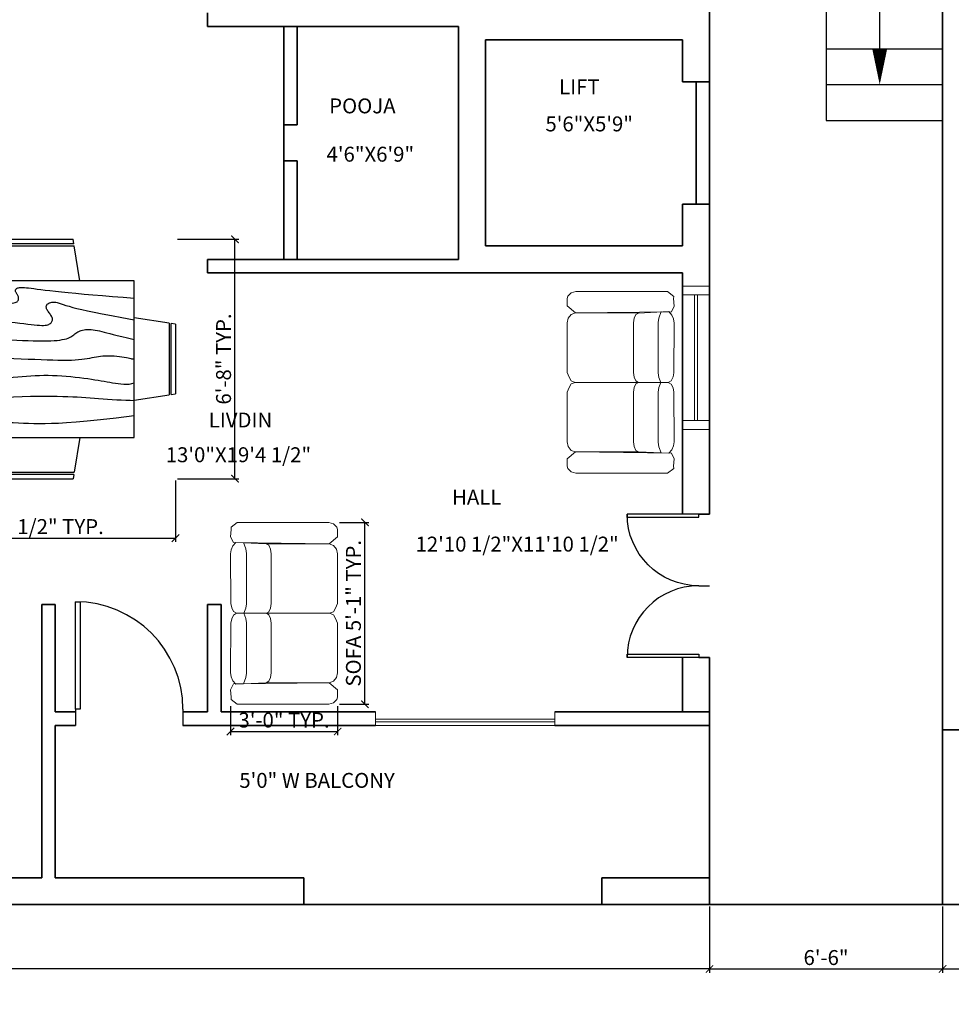
# Model space of a CAD drawing. Units: inches. Extents: x 3283068 to 3284536, y 3240756 to 3241803.
# Tile 14 of 19: x 3283598 to 3283910, y 3241165 to 3241494. Entities that reach past the tile are written whole.
import ezdxf

# ---------------------------------------------------------------- set-up
doc = ezdxf.new("R2010")
doc.units = ezdxf.units.IN
for name, color, linetype, lineweight in [('A-ANNO-DIMS', 2, 'Continuous', 18), ('A-AREA-IDEN', 7, 'Continuous', 18), ('door', 140, 'Continuous', 25), ('furniture', 40, 'Continuous', 18), ('STAIR', 50, 'Continuous', 25), ('wall', 20, 'Continuous', 35), ('window', 100, 'Continuous', 18)]:
    doc.layers.add(name, color=color, linetype=linetype, lineweight=lineweight)
doc.layers.add('HATCH', color=8, linetype='Continuous')
doc.layers.add('NOI THAT', color=42, linetype='Continuous')
doc.styles.get("Standard").update_dxf_attribs({"font": 'arial.ttf'})
doc.dimstyles.new('ISO-25', dxfattribs={"dimtxt": 5, "dimasz": 2.5, "dimexe": 1.25, "dimexo": 0.625, "dimtad": 1, "dimlunit": 4, "dimtxsty": 'Standard', "dimblk": 'ARCHTICK', "dimcen": 2.5, "dimadec": 0, "dimazin": 0, "dimtfac": 1, "dimtmove": 0, "dimatfit": 3, "dimfxl": 1, "dimarcsym": 0})

# ---------------------------------------------------------------- blocks, each defined once
blk = doc.blocks.new('*U3')
for p, q in [((0, 0), (0, -6)), ((40, 0), (40, -6))]:
    blk.add_line(p, q)
blk.add_lwpolyline([(0, 0), (0, 40), (1.75, 40), (1.75, 0)], close=True)
blk.add_arc((0, 0), 40, 0, 90)
blk = doc.blocks.new('*U4')
for p, q in [((-40, 0), (-40, 6)), ((0, 0), (0, 6))]:
    blk.add_line(p, q)
blk.add_lwpolyline([(0, 0), (0, -40), (-1.75, -40), (-1.75, 0)], close=True)
blk.add_arc((0, 0), 40, 180, 270)
blk = doc.blocks.new('A$C78170A85')
at = {"layer": 'HATCH'}
for points in [[(171.5, 767.4), (258.6, 767), (337.5, 765.8), (408.9, 764), (473.5, 761.7), (532, 759), (585.1, 755.9), (633.5, 752.7), (677.8, 749.3), (718.8, 745.9), (756.5, 742.6), (790.9, 739.5), (822.2, 736.5), (850.3, 733.8), (875.4, 731.5), (897.3, 729.6), (916.3, 728.2), (932.4, 727.4), (945.8, 727.1), (956.7, 727.2), (965.6, 727.9), (972.6, 728.9), (978.1, 730.4), (982.3, 732.1), (985.5, 734.3), (988, 736.6), (989.8, 739.3), (991.1, 742.1), (991.7, 745), (991.9, 748), (991.7, 751), (991, 753.9), (990, 756.8), (988.8, 759.6), (987.3, 762.2), (985.8, 764.7), (984.2, 767.2), (982.7, 769.5), (981.4, 771.9), (980.3, 774.1), (979.5, 776.4), (979.2, 778.6), (979.2, 780.9), (979.7, 783), (980.6, 785), (982, 786.9), (983.7, 788.7), (985.9, 790.2), (988.5, 791.4), (991.6, 792.4), (995.2, 793.1), (999.4, 793.6), (1004.3, 793.7), (1010.1, 793.6), (1016.9, 793.1), (1024.7, 792.4), (1033.7, 791.4), (1043.9, 790.2), (1055.7, 788.6), (1069.2, 786.9), (1084.6, 784.9), (1102.1, 782.6), (1122, 780.2), (1144.5, 777.6), (1169.9, 774.9), (1198.1, 772), (1229.4, 769), (1263.4, 765.9), (1300.1, 762.7), (1339.4, 759.4), (1381.1, 756.1), (1425.2, 752.7), (1471.5, 749.3)], [(171.5, 677.1), (298.3, 679.7), (403.1, 680.8), (488.9, 680.7), (558.5, 679.5), (615, 677.6), (661.2, 675.2), (700.3, 672.4), (735, 669.6), (767.9, 666.8), (799.4, 664.2), (829.5, 661.7), (858.1, 659.2), (885.2, 656.9), (910.7, 654.5), (934.7, 652.3), (956.9, 650), (977.5, 647.8), (996.5, 645.6), (1013.9, 643.5), (1029.7, 641.5), (1044.1, 639.8), (1057, 638.4), (1068.6, 637.2), (1078.8, 636.5), (1087.8, 636.1), (1095.6, 636.2), (1102.4, 636.6), (1108.2, 637.4), (1113.1, 638.6), (1117.3, 640.1), (1120.9, 641.9), (1124, 644), (1126.6, 646.4), (1128.7, 649), (1130.4, 651.9), (1131.7, 654.9), (1132.4, 658.1), (1132.6, 661.3), (1132.3, 664.7), (1131.5, 668.1), (1130.1, 671.4), (1128.2, 674.8), (1126, 678.2), (1123.6, 681.6), (1121, 685), (1118.4, 688.4), (1115.8, 691.8), (1113.4, 695.1), (1111.3, 698.5), (1109.5, 701.9), (1108.2, 705.2), (1107.2, 708.5), (1106.8, 711.7), (1106.9, 714.8), (1107.6, 717.8), (1108.9, 720.7), (1110.9, 723.5), (1113.6, 726), (1116.9, 728.2), (1120.8, 730.1), (1125.1, 731.6), (1129.9, 732.6), (1135, 733), (1140.5, 732.8), (1146.3, 731.8), (1152.7, 730.3), (1159.9, 728.2), (1168.1, 725.5), (1177.6, 722.4), (1188.6, 718.9), (1201.5, 715.1), (1216.5, 710.9), (1233.8, 706.6), (1254.1, 701.9), (1277.9, 696.7), (1305.9, 690.9), (1338.7, 684.4), (1376.8, 677), (1420.9, 668.6), (1471.5, 659)], [(171.5, 595.8), (266.9, 592.9), (350.8, 590.6), (424.4, 588.9), (488.8, 587.7), (545.3, 586.9), (594.9, 586.3), (639, 585.8), (678.6, 585.3), (714.8, 584.7), (748.2, 583.9), (779.2, 583.1), (808.2, 582.1), (835.5, 581.1), (861.6, 580), (886.9, 578.9), (911.8, 577.8), (936.6, 576.7), (961.2, 575.6), (985.3, 574.6), (1008.9, 573.6), (1031.5, 572.9), (1053.1, 572.3), (1073.5, 571.9), (1092.4, 571.8), (1109.6, 571.9), (1125.2, 572.3), (1139.3, 573), (1152, 574), (1163.3, 575.3), (1173.4, 576.8), (1182.3, 578.7), (1190.2, 580.8), (1197, 583.2), (1203, 585.8), (1208.4, 588.6), (1213.1, 591.5), (1217.4, 594.5), (1221.5, 597.5), (1225.4, 600.5), (1229.3, 603.4), (1233.3, 606.1), (1237.5, 608.7), (1242, 611), (1246.8, 613.1), (1251.9, 615), (1257.4, 616.5), (1263.4, 617.6), (1269.9, 618.4), (1277, 618.8), (1284.5, 618.7), (1292.5, 618.3), (1300.9, 617.5), (1309.7, 616.3), (1318.8, 614.8), (1328.1, 613), (1337.6, 610.9), (1347.4, 608.5), (1357.9, 605.7), (1369.8, 602.5), (1383.7, 598.8), (1400.2, 594.6), (1419.9, 589.7), (1443.5, 584.1), (1471.5, 577.8)], [(171.5, 478.5), (265.6, 484.6), (351.7, 489.6), (430.6, 493.6), (502.7, 496.6), (568.7, 498.8), (629.2, 500.4), (684.7, 501.3), (735.8, 501.8), (783, 501.9), (826.7, 501.7), (867.2, 501.3), (904.8, 500.6), (939.8, 499.7), (972.5, 498.7), (1003.2, 497.6), (1032.2, 496.5), (1059.7, 495.4), (1085.8, 494.3), (1110.4, 493.4), (1133.6, 492.6), (1155.2, 492), (1175.4, 491.7), (1194.1, 491.7), (1211.2, 492), (1226.8, 492.8), (1241.1, 493.9), (1254, 495.3), (1266, 496.9), (1277, 498.7), (1287.2, 500.5), (1296.8, 502.3), (1306, 504.1), (1314.9, 505.7), (1323.7, 507.1), (1332.3, 508.3), (1341, 509.3), (1349.8, 510), (1358.9, 510.4), (1368.3, 510.4), (1378.2, 510.1), (1388.6, 509.3), (1399.3, 508.2), (1409.9, 506.9), (1420.3, 505.4), (1430, 503.8), (1438.9, 502.2), (1446.5, 500.8), (1452.7, 499.5), (1457.3, 498.5), (1460.4, 497.8), (1462.6, 497.3), (1464.1, 496.9), (1465.4, 496.7), (1466.8, 496.6), (1468.7, 496.5), (1471.5, 496.5)], [(171.5, 379.2), (330.7, 382.5), (458.9, 385.9), (560.3, 389.2), (639, 392.5), (699.2, 395.7), (745, 398.8), (780.7, 401.9), (810.2, 404.7), (837.3, 407.5), (862.5, 410.1), (886.3, 412.6), (908.7, 414.9), (929.9, 417.1), (950.2, 419.1), (969.7, 421), (988.5, 422.8), (1007, 424.4), (1025.1, 425.9), (1043, 427.1), (1060.8, 428.1), (1078.6, 428.8), (1096.5, 429.1), (1114.6, 429.2), (1133, 428.8), (1151.8, 428.1), (1170.8, 426.9), (1189.9, 425.5), (1208.8, 423.7), (1227.3, 421.8), (1245.3, 419.7), (1262.6, 417.5), (1278.9, 415.3), (1294.2, 413), (1308.5, 410.8), (1321.9, 408.5), (1334.7, 406.3), (1346.9, 404.2), (1358.8, 402.1), (1370.4, 400), (1382, 398), (1393.6, 396.1), (1405.2, 394.4), (1416.7, 393), (1428.2, 392.2), (1439.4, 392.1), (1450.5, 392.8), (1461.2, 394.4), (1471.5, 397.2)], [(171.5, 316), (344.8, 319.3), (488.1, 322.7), (605.2, 325.9), (699.8, 328.9), (776, 331.8), (837.4, 334.4), (887.9, 336.6), (931.4, 338.5), (971, 340), (1007.5, 341.1), (1041.3, 341.9), (1072.4, 342.3), (1101.2, 342.5), (1127.7, 342.4), (1152.3, 342), (1175.1, 341.6), (1196.4, 340.9), (1216.4, 340.2), (1235.3, 339.3), (1253.5, 338.3), (1271.3, 337.2), (1288.7, 335.9), (1306.3, 334.6), (1324.1, 333.3), (1342.4, 331.8), (1361.1, 330.4), (1380, 329), (1398.9, 327.7), (1417.7, 326.6), (1436.2, 325.8), (1454.2, 325.2), (1471.5, 325)], [(171.5, 234.7), (278.3, 237.7), (369.5, 239.9), (447.2, 241.5), (513.2, 242.4), (569.3, 242.9), (617.5, 243), (659.5, 242.7), (697.4, 242.2), (732.7, 241.6), (765.7, 240.9), (796.8, 240), (825.9, 239), (853.4, 238), (879.3, 237), (903.7, 235.8), (926.9, 234.7), (948.9, 233.6), (970.2, 232.5), (991.1, 231.5), (1012, 230.7), (1033.1, 230), (1055, 229.5), (1077.9, 229.3), (1102.1, 229.5), (1128.4, 230), (1157.6, 231), (1191.3, 232.9), (1230.7, 235.8), (1277.1, 239.9), (1331.8, 245.4), (1396.2, 252.7), (1471.5, 261.8)]]:
    blk.add_lwpolyline(points, dxfattribs=at)
at = {"layer": 'NOI THAT'}
for p, q in [((424.3, 993.1), (421.5, 975)), ((424.3, 993.1), (713.2, 993.1)), ((716, 975), (713.2, 993.1)), ((929.9, 993.1), (927, 975)), ((929.9, 993.1), (1218.8, 993.1)), ((1221.6, 975), (1218.8, 993.1)), ((420.1, 966), (397.5, 821.5)), ((420.1, 966), (717.5, 966)), ((716.1, 975), (421.5, 975)), ((740, 821.5), (717.4, 966)), ((925.6, 966), (903.1, 821.5)), ((925.7, 966), (1223.1, 966)), ((1221.6, 975), (927.1, 975)), ((1245.6, 821.5), (1223, 966)), ((1471.5, 821.5), (171.5, 821.5)), ((171.5, 821.5), (171.5, 171.5)), ((1471.5, 171.5), (1471.5, 821.5)), ((27.1, 645.2), (171.6, 667.8)), ((1616, 645.2), (1471.5, 667.8)), ((0, 641), (18, 643.8)), ((0, 641), (0, 352.1)), ((18.1, 349.2), (18.1, 643.7)), ((27.1, 645.1), (27.1, 347.8)), ((1616, 645.1), (1616, 347.8)), ((1643.1, 641), (1625, 643.8)), ((1625, 349.2), (1625, 643.7)), ((1643.1, 641), (1643.1, 352.1)), ((18.1, 349.3), (0, 352.1)), ((171.6, 325.3), (27.1, 347.8)), ((1471.5, 325.3), (1616, 347.8)), ((1625, 349.3), (1643.1, 352.1)), ((420.1, 27.1), (397.5, 171.6)), ((740, 171.6), (717.4, 27.1)), ((925.6, 27.1), (903.1, 171.6)), ((1245.6, 171.6), (1223, 27.1)), ((420.1, 27.1), (717.5, 27.1)), ((716.1, 18.1), (421.5, 18.1)), ((424.3, 0), (421.5, 18)), ((424.3, 0), (713.2, 0)), ((716, 18.1), (713.2, 0)), ((925.7, 27.1), (1223.1, 27.1)), ((929.9, 0), (927, 18)), ((1221.6, 18.1), (927.1, 18.1)), ((929.9, 0), (1218.8, 0)), ((1221.6, 18.1), (1218.8, 0))]:
    blk.add_line(p, q, dxfattribs=at)
at = {"layer": 'NOI THAT', "ltscale": 20}
blk.add_line((171.5, 171.5), (1471.5, 171.5), dxfattribs=at)
blk = doc.blocks.new('12PCOU16')
at = {"color": 0, "linetype": 'ByBlock'}
for points in [[(-33.06, 29.95), (-35.14, 28.36), (-35.08, 27.62), (-35.3, 25.17), (-34.36, 23.28), (-2.78, 22.92), (-0.03, 25.21), (-0.03, 27.62), (-0.03, 27.62), (-0.26, 28.4), (-1.38, 29.51), (-2.93, 29.96), (-33.06, 29.95)], [(-30.87, 0), (-30.25, 1.66), (-30.05, 3.17), (-30.05, 19.69), (-30.25, 21.21), (-31.05, 23.33)], [(-23.5, 0), (-2.65, 0), (-1.32, 0.48), (-0.72, 1.72), (0, 3.25), (0, 3.25), (0, 19.62), (-0.39, 21.14), (-1.32, 22.39), (-2.78, 22.92), (-23.51, 22.87)], [(-30.87, 0), (-30.25, -1.66), (-30.05, -3.17), (-30.05, -19.69), (-30.25, -21.21), (-31, -23.21)], [(-23.5, 0), (-2.65, 0), (-1.32, -0.48), (-0.72, -1.72), (0, -3.25), (0, -3.25), (0, -19.62), (-0.39, -21.14), (-1.32, -22.39), (-2.78, -22.92), (-23.51, -22.87)], [(-33.06, -29.95), (-35.14, -28.36), (-35.08, -27.62), (-35.3, -25.17), (-34.36, -23.28), (-2.78, -22.92), (-0.03, -25.21), (-0.03, -27.62), (-0.03, -27.62), (-0.26, -28.4), (-1.38, -29.51), (-2.93, -29.96), (-33.06, -29.95)]]:
    blk.add_lwpolyline(points, dxfattribs=at)
for points in [[(-23.5, 0), (-22.65, 0.47), (-22.11, 1.72), (-21.88, 3.23), (-21.88, 19.63), (-22.11, 21.15), (-22.65, 22.4), (-23.51, 22.87), (-33.55, 23.32), (-34.49, 22.2), (-35.08, 20.94), (-35.33, 19.56), (-35.15, 3.2), (-34.9, 1.81), (-34.31, 0.56), (-33.28, 0)], [(-23.5, 0), (-22.65, -0.47), (-22.11, -1.72), (-21.88, -3.23), (-21.88, -19.63), (-22.11, -21.15), (-22.65, -22.4), (-23.51, -22.87), (-33.55, -23.32), (-34.49, -22.2), (-35.08, -20.94), (-35.33, -19.56), (-35.15, -3.2), (-34.9, -1.81), (-34.31, -0.56), (-33.28, 0)]]:
    blk.add_lwpolyline(points, close=True, dxfattribs=at)
blk = doc.blocks.new('_ArchTick')
at = {"color": 0, "linetype": 'ByBlock', "const_width": 0.15}
blk.add_lwpolyline([(-0.5, -0.5), (0.5, 0.5)], dxfattribs=at)
blk = doc.blocks.new('*D27')
at = {"layer": 'A-ANNO-DIMS', "color": 0, "lineweight": -2, "transparency": 16777216}
for p, q in [((3283828.59, 3241197.48), (3283828.59, 3241175.31)), ((3283906.59, 3241197.48), (3283906.59, 3241175.31)), ((3283828.59, 3241176.56), (3283906.59, 3241176.56))]:
    blk.add_line(p, q, dxfattribs=at)
at = {"layer": 'Defpoints', "color": 0, "transparency": 16777216}
for p in [(3283828.59, 3241198.1), (3283906.59, 3241198.1), (3283906.59, 3241176.56)]:
    blk.add_point(p, dxfattribs=at)
at = {"layer": 'A-ANNO-DIMS', "color": 0, "lineweight": -2, "transparency": 16777216, "xscale": 2.5, "yscale": 2.5, "zscale": 2.5, "rotation": 180}
blk.add_blockref('_ArchTick', (3283828.59, 3241176.56), dxfattribs=at)
at = {"layer": 'A-ANNO-DIMS', "color": 0, "lineweight": -2, "transparency": 16777216, "xscale": 2.5, "yscale": 2.5, "zscale": 2.5}
blk.add_blockref('_ArchTick', (3283906.59, 3241176.56), dxfattribs=at)
at = {"layer": 'A-ANNO-DIMS', "color": 0, "transparency": 16777216, "insert": (3283867.59, 3241179.74), "char_height": 5, "attachment_point": 5}
blk.add_mtext('6\'-6"', dxfattribs=at)
blk = doc.blocks.new('*D28')
at = {"layer": 'A-ANNO-DIMS', "color": 0, "lineweight": -2, "transparency": 16777216}
for p, q in [((3283906.59, 3241197.48), (3283906.59, 3241175.31)), ((3284236.59, 3241197.48), (3284236.59, 3241175.31)), ((3283906.59, 3241176.56), (3284236.59, 3241176.56))]:
    blk.add_line(p, q, dxfattribs=at)
at = {"layer": 'Defpoints', "color": 0, "transparency": 16777216}
for p in [(3283906.59, 3241198.1), (3284236.59, 3241198.1), (3284236.59, 3241176.56)]:
    blk.add_point(p, dxfattribs=at)
at = {"layer": 'A-ANNO-DIMS', "color": 0, "lineweight": -2, "transparency": 16777216, "xscale": 2.5, "yscale": 2.5, "zscale": 2.5, "rotation": 180}
blk.add_blockref('_ArchTick', (3283906.59, 3241176.56), dxfattribs=at)
at = {"layer": 'A-ANNO-DIMS', "color": 0, "lineweight": -2, "transparency": 16777216, "xscale": 2.5, "yscale": 2.5, "zscale": 2.5}
blk.add_blockref('_ArchTick', (3284236.59, 3241176.56), dxfattribs=at)
at = {"layer": 'A-ANNO-DIMS', "color": 0, "transparency": 16777216, "insert": (3284071.59, 3241179.74), "char_height": 5, "attachment_point": 5}
blk.add_mtext('27\'-6"', dxfattribs=at)
blk = doc.blocks.new('*D29')
at = {"layer": 'A-ANNO-DIMS', "color": 0, "lineweight": -2, "transparency": 16777216}
for p, q in [((3283339.59, 3241197.48), (3283339.59, 3241175.31)), ((3283828.59, 3241197.48), (3283828.59, 3241175.31)), ((3283828.59, 3241176.56), (3283339.59, 3241176.56))]:
    blk.add_line(p, q, dxfattribs=at)
at = {"layer": 'Defpoints', "color": 0, "transparency": 16777216}
for p in [(3283339.59, 3241198.1), (3283828.59, 3241198.1), (3283339.59, 3241176.56)]:
    blk.add_point(p, dxfattribs=at)
at = {"layer": 'A-ANNO-DIMS', "color": 0, "lineweight": -2, "transparency": 16777216, "xscale": 2.5, "yscale": 2.5, "zscale": 2.5, "rotation": 180}
blk.add_blockref('_ArchTick', (3283339.59, 3241176.56), dxfattribs=at)
at = {"layer": 'A-ANNO-DIMS', "color": 0, "lineweight": -2, "transparency": 16777216, "xscale": 2.5, "yscale": 2.5, "zscale": 2.5}
blk.add_blockref('_ArchTick', (3283828.59, 3241176.56), dxfattribs=at)
at = {"layer": 'A-ANNO-DIMS', "color": 0, "transparency": 16777216, "insert": (3283584.09, 3241179.74), "char_height": 5, "attachment_point": 5}
blk.add_mtext('40\'-9"', dxfattribs=at)
blk = doc.blocks.new('WIN-48IN-9IN-WALL')
for p, q in [((0, 9), (48, 9)), ((0, 0), (0, 9)), ((3, 0), (3, 9)), ((45, 9), (45, 0)), ((48, 9), (48, 0)), ((3, 5), (45, 5)), ((3, 4), (45, 4)), ((48, 0), (0, 0))]:
    blk.add_line(p, q)
blk = doc.blocks.new('*D53')
at = {"layer": 'A-ANNO-DIMS', "color": 0, "lineweight": -2, "transparency": 16777216}
for p, q in [((3283517.27, 3241340.06), (3283517.27, 3241319.55)), ((3283649.87, 3241340.06), (3283649.87, 3241319.55)), ((3283517.27, 3241320.8), (3283649.87, 3241320.8))]:
    blk.add_line(p, q, dxfattribs=at)
at = {"layer": 'Defpoints', "color": 0, "transparency": 16777216}
for p in [(3283517.27, 3241340.69), (3283649.87, 3241340.69), (3283649.87, 3241320.8)]:
    blk.add_point(p, dxfattribs=at)
at = {"layer": 'A-ANNO-DIMS', "color": 0, "lineweight": -2, "transparency": 16777216, "xscale": 2.5, "yscale": 2.5, "zscale": 2.5, "rotation": 180}
blk.add_blockref('_ArchTick', (3283517.27, 3241320.8), dxfattribs=at)
at = {"layer": 'A-ANNO-DIMS', "color": 0, "lineweight": -2, "transparency": 16777216, "xscale": 2.5, "yscale": 2.5, "zscale": 2.5}
blk.add_blockref('_ArchTick', (3283649.87, 3241320.8), dxfattribs=at)
at = {"layer": 'A-ANNO-DIMS', "color": 0, "transparency": 16777216, "insert": (3283583.57, 3241324.01), "char_height": 5, "attachment_point": 5}
blk.add_mtext('DINING SET 11\'-0 1/2" TYP.', dxfattribs=at)
blk = doc.blocks.new('*D54')
at = {"layer": 'A-ANNO-DIMS', "color": 0, "lineweight": -2, "transparency": 16777216}
for p, q in [((3283650.5, 3241420.83), (3283671.01, 3241420.83)), ((3283669.76, 3241340.69), (3283669.76, 3241420.83)), ((3283650.5, 3241340.69), (3283671.01, 3241340.69))]:
    blk.add_line(p, q, dxfattribs=at)
at = {"layer": 'Defpoints', "color": 0, "transparency": 16777216}
for p in [(3283649.87, 3241420.83), (3283669.76, 3241420.83), (3283649.87, 3241340.69)]:
    blk.add_point(p, dxfattribs=at)
at = {"layer": 'A-ANNO-DIMS', "color": 0, "lineweight": -2, "transparency": 16777216, "xscale": 2.5, "yscale": 2.5, "zscale": 2.5}
for p, rotation in [((3283669.76, 3241420.83), 90), ((3283669.76, 3241340.69), 270)]:
    blk.add_blockref('_ArchTick', p, dxfattribs=dict(at, rotation=rotation))
at = {"layer": 'A-ANNO-DIMS', "color": 0, "transparency": 16777216, "insert": (3283666.58, 3241380.76), "char_height": 5, "attachment_point": 5, "rotation": 90}
blk.add_mtext('6\'-8" TYP.', dxfattribs=at)
blk = doc.blocks.new('*D55')
at = {"layer": 'A-ANNO-DIMS', "color": 0, "lineweight": -2, "transparency": 16777216}
for p, q in [((3283704.75, 3241326.07), (3283714.51, 3241326.07)), ((3283713.26, 3241265.19), (3283713.26, 3241326.07)), ((3283704.75, 3241265.19), (3283714.51, 3241265.19))]:
    blk.add_line(p, q, dxfattribs=at)
at = {"layer": 'Defpoints', "color": 0, "transparency": 16777216}
for p in [(3283704.13, 3241326.07), (3283713.26, 3241326.07), (3283704.13, 3241265.19)]:
    blk.add_point(p, dxfattribs=at)
at = {"layer": 'A-ANNO-DIMS', "color": 0, "lineweight": -2, "transparency": 16777216, "xscale": 2.5, "yscale": 2.5, "zscale": 2.5}
for p, rotation in [((3283713.26, 3241326.07), 90), ((3283713.26, 3241265.19), 270)]:
    blk.add_blockref('_ArchTick', p, dxfattribs=dict(at, rotation=rotation))
at = {"layer": 'A-ANNO-DIMS', "color": 0, "transparency": 16777216, "insert": (3283710.05, 3241295.63), "char_height": 5, "attachment_point": 5, "rotation": 90}
blk.add_mtext('SOFA 5\'-1" TYP.', dxfattribs=at)
blk = doc.blocks.new('*D56')
at = {"layer": 'A-ANNO-DIMS', "color": 0, "lineweight": -2, "transparency": 16777216}
for p, q in [((3283668.24, 3241264.57), (3283668.24, 3241254.81)), ((3283704.13, 3241264.57), (3283704.13, 3241254.81)), ((3283668.24, 3241256.06), (3283704.13, 3241256.06))]:
    blk.add_line(p, q, dxfattribs=at)
at = {"layer": 'Defpoints', "color": 0, "transparency": 16777216}
for p in [(3283668.24, 3241265.19), (3283704.13, 3241265.19), (3283704.13, 3241256.06)]:
    blk.add_point(p, dxfattribs=at)
at = {"layer": 'A-ANNO-DIMS', "color": 0, "lineweight": -2, "transparency": 16777216, "xscale": 2.5, "yscale": 2.5, "zscale": 2.5, "rotation": 180}
blk.add_blockref('_ArchTick', (3283668.24, 3241256.06), dxfattribs=at)
at = {"layer": 'A-ANNO-DIMS', "color": 0, "lineweight": -2, "transparency": 16777216, "xscale": 2.5, "yscale": 2.5, "zscale": 2.5}
blk.add_blockref('_ArchTick', (3283704.13, 3241256.06), dxfattribs=at)
at = {"layer": 'A-ANNO-DIMS', "color": 0, "transparency": 16777216, "insert": (3283686.18, 3241259.24), "char_height": 5, "attachment_point": 5}
blk.add_mtext('3\'-0" TYP.', dxfattribs=at)
blk = doc.blocks.new('*D63')
at = {"layer": 'A-ANNO-DIMS', "color": 0, "lineweight": -2, "transparency": 16777216}
for p, q in [((3283248.09, 3241083.23), (3283248.09, 3241798.08)), ((3284328.09, 3241083.23), (3284328.09, 3241798.08)), ((3283248.09, 3241796.83), (3284328.09, 3241796.83))]:
    blk.add_line(p, q, dxfattribs=at)
at = {"layer": 'Defpoints', "color": 0, "transparency": 16777216}
for p in [(3284328.09, 3241796.83), (3283248.09, 3241082.6), (3284328.09, 3241082.6)]:
    blk.add_point(p, dxfattribs=at)
at = {"layer": 'A-ANNO-DIMS', "color": 0, "lineweight": -2, "transparency": 16777216, "xscale": 2.5, "yscale": 2.5, "zscale": 2.5, "rotation": 180}
blk.add_blockref('_ArchTick', (3283248.09, 3241796.83), dxfattribs=at)
at = {"layer": 'A-ANNO-DIMS', "color": 0, "lineweight": -2, "transparency": 16777216, "xscale": 2.5, "yscale": 2.5, "zscale": 2.5}
blk.add_blockref('_ArchTick', (3284328.09, 3241796.83), dxfattribs=at)
at = {"layer": 'A-ANNO-DIMS', "color": 0, "transparency": 16777216, "insert": (3283788.09, 3241800.01), "char_height": 5, "attachment_point": 5}
blk.add_mtext('90\'-0"', dxfattribs=at)

msp = doc.modelspace()

# ---------------------------------------------------------------- linework, layer by layer
at = {"layer": 'door'}
for p, q in [((3283828.589, 3241328.853), (3283819.589, 3241328.853)), ((3283828.589, 3241280.853), (3283819.589, 3241280.853)), ((3283616.326, 3241262.602), (3283616.326, 3241258.102)), ((3283652.326, 3241262.602), (3283652.326, 3241258.102))]:
    msp.add_line(p, q, dxfattribs=at)
at = {"layer": 'STAIR'}
for p, q in [((3283885.56, 3241484.602), (3283885.56, 3241610.107)), ((3283867.589, 3241604.602), (3283867.589, 3241460.602)), ((3283867.589, 3241484.602), (3283906.589, 3241484.602)), ((3283867.589, 3241472.602), (3283906.589, 3241472.602)), ((3283867.589, 3241460.602), (3283906.589, 3241460.602))]:
    msp.add_line(p, q, dxfattribs=at)
msp.add_lwpolyline([(3283885.56, 3241484.602, 5, 0, 0), (3283885.56, 3241472.602, 0, 0, 0)], format="xyseb", dxfattribs=at)
at = {"layer": 'wall'}
for p, q in [((3283828.589, 3241630.102), (3283828.589, 3241328.853)), ((3283906.589, 3241630.102), (3283906.589, 3241198.102)), ((3283660.589, 3241496.602), (3283660.589, 3241492.102)), ((3283744.589, 3241492.102), (3283660.589, 3241492.102)), ((3283686.089, 3241492.102), (3283686.089, 3241414.102)), ((3283690.589, 3241492.102), (3283690.589, 3241459.102)), ((3283744.589, 3241492.102), (3283744.589, 3241414.102)), ((3283753.589, 3241487.602), (3283753.589, 3241418.602)), ((3283753.589, 3241487.602), (3283819.589, 3241487.602)), ((3283819.589, 3241487.602), (3283819.589, 3241473.57)), ((3283819.589, 3241473.57), (3283828.589, 3241473.57)), ((3283824.089, 3241473.57), (3283824.089, 3241432.635)), ((3283690.589, 3241459.102), (3283686.089, 3241459.102)), ((3283690.589, 3241447.102), (3283686.089, 3241447.102)), ((3283690.589, 3241447.102), (3283690.589, 3241414.102)), ((3283819.589, 3241432.635), (3283828.589, 3241432.635)), ((3283819.589, 3241418.602), (3283819.589, 3241432.635)), ((3283753.589, 3241418.602), (3283819.589, 3241418.602)), ((3283660.589, 3241414.102), (3283744.589, 3241414.102)), ((3283660.589, 3241414.102), (3283660.589, 3241409.602)), ((3283660.589, 3241409.602), (3283819.589, 3241409.602)), ((3283819.589, 3241328.853), (3283819.589, 3241409.602)), ((3283605.089, 3241207.102), (3283605.089, 3241298.602)), ((3283605.089, 3241298.602), (3283609.589, 3241298.602)), ((3283609.589, 3241262.602), (3283609.589, 3241298.602)), ((3283660.589, 3241262.602), (3283660.589, 3241298.602)), ((3283660.589, 3241298.602), (3283665.089, 3241298.602)), ((3283665.089, 3241262.602), (3283665.089, 3241298.602)), ((3283819.589, 3241262.602), (3283819.589, 3241280.853)), ((3283828.589, 3241280.853), (3283828.589, 3241198.102)), ((3283609.589, 3241262.602), (3283616.326, 3241262.602)), ((3283652.326, 3241262.602), (3283660.589, 3241262.602)), ((3283665.089, 3241262.602), (3283716.839, 3241262.602)), ((3283776.839, 3241262.602), (3283828.589, 3241262.602)), ((3283609.589, 3241207.102), (3283609.589, 3241258.102)), ((3283609.589, 3241258.102), (3283616.326, 3241258.102)), ((3283652.326, 3241258.102), (3283716.839, 3241258.102)), ((3283776.839, 3241258.102), (3283828.589, 3241258.102)), ((3283906.589, 3241256.602), (3284189.004, 3241256.602)), ((3283461.089, 3241207.102), (3283605.089, 3241207.102)), ((3283609.589, 3241207.102), (3283692.814, 3241207.102)), ((3283692.814, 3241207.102), (3283692.814, 3241198.102)), ((3283792.589, 3241207.102), (3283828.589, 3241207.102)), ((3283792.589, 3241207.102), (3283792.589, 3241198.102)), ((3283339.589, 3241198.102), (3284236.589, 3241198.102))]:
    msp.add_line(p, q, dxfattribs=at)
at = {"layer": 'window'}
for p, q in [((3283716.839, 3241262.602), (3283716.839, 3241258.102)), ((3283776.839, 3241258.102), (3283776.839, 3241262.602)), ((3283716.839, 3241260.219), (3283776.839, 3241260.219)), ((3283716.839, 3241259.283), (3283776.839, 3241259.283)), ((3283716.839, 3241258.102), (3283776.839, 3241258.102))]:
    msp.add_line(p, q, dxfattribs=at)

# ---------------------------------------------------------------- block references
at = {"layer": 'door', "yscale": 0.5999999999973883, "zscale": 0.5999999999973883}
for p, xscale, rotation in [((3283824.989, 3241328.853), -0.5999999999973883, 270), ((3283824.989, 3241280.853), 0.5999999999973883, 269.9999999999999)]:
    msp.add_blockref('*U4', p, dxfattribs=dict(at, xscale=xscale, rotation=rotation))
at = {"layer": 'door', "xscale": 0.9, "yscale": 0.9, "zscale": 0.9}
msp.add_blockref('*U3', (3283616.326, 3241263.502), dxfattribs=at)
at = {"layer": 'furniture'}
for name, p, xscale, yscale, zscale in [('A$C78170A85', (3283517.269, 3241340.686), 0.0807042311318891, 0.0807042311318891, 0.0807042311318891), ('12PCOU16', (3283780.921, 3241372.929), -1.01584888439622, 1.01584888439622, 1.01584888439622), ('12PCOU16', (3283704.13, 3241295.629), 1.01584888439622, 1.01584888439622, 1.01584888439622)]:
    msp.add_blockref(name, p, dxfattribs=dict(at, xscale=xscale, yscale=yscale, zscale=zscale))
at = {"layer": 'window', "rotation": 269.999999998322}
msp.add_blockref('WIN-48IN-9IN-WALL', (3283819.589, 3241405.193), dxfattribs=at)

# ---------------------------------------------------------------- texts
at = {"layer": 'A-AREA-IDEN'}
for s, p in [('   LIFT', (3283773.663, 3241469.35)), ('POOJA', (3283701.289, 3241462.995)), ('5\'6"X5\'9"', (3283773.663, 3241456.959)), ('4\'6"X6\'9"', (3283700.409, 3241446.822)), ('LIVDIN', (3283660.98, 3241357.833)), ('13\'0"X19\'4 1/2"', (3283646.588, 3241346.211)), ('        HALL', (3283730.198, 3241332.027)), ('12\'10 1/2"X11\'10 1/2"', (3283730.198, 3241316.292))]:
    msp.add_text(s, height=5, dxfattribs=at).set_placement(p)
at = {"layer": 'A-AREA-IDEN', "insert": (3283671.213, 3241242.195), "char_height": 5, "attachment_point": 1}
msp.add_mtext_dynamic_manual_height_columns('5\'0" W BALCONY', width=85.09051, gutter_width=12.5, heights=[0], dxfattribs=at)

# ---------------------------------------------------------------- dimensions: what is measured, and where the dimension line sits
at = {"layer": 'A-ANNO-DIMS'}
for base, p1, p2, override, picture, middle in [((3284328.089, 3241796.827), (3283248.089, 3241082.602), (3284328.089, 3241082.602), {"dimdec": 1, "dimlfac": 1, "dimrnd": 0, "dimzin": 1, "dimdsep": 46, "dimlunit": 4, "dimfrac": 2}, '*D63', (3283788.089, 3241800.005)), ((3283339.589, 3241176.561), (3283828.589, 3241198.102), (3283339.589, 3241198.102), {"dimclrd": 0, "dimclre": 0, "dimclrt": 0}, '*D29', (3283584.089, 3241179.739)), ((3283906.589, 3241176.561), (3283828.589, 3241198.102), (3283906.589, 3241198.102), {"dimclrd": 0, "dimclre": 0, "dimclrt": 0}, '*D27', (3283867.589, 3241179.739)), ((3284236.589, 3241176.561), (3283906.589, 3241198.102), (3284236.589, 3241198.102), {"dimclrd": 0, "dimclre": 0, "dimclrt": 0, "dimtmove": 1}, '*D28', (3284071.589, 3241179.739))]:
    dim = msp.add_linear_dim(base=base, p1=p1, p2=p2, dimstyle='ISO-25', override=override, dxfattribs=at)
    dim.commit()
    dim.dimension.update_dxf_attribs({"geometry": picture, "text_midpoint": middle})
for base, p1, p2, text, picture, middle in [((3283669.761, 3241420.83), (3283649.87, 3241340.686), (3283649.87, 3241420.83), '<> TYP.', '*D54', (3283666.583, 3241380.758)), ((3283713.261, 3241326.066), (3283704.13, 3241265.193), (3283704.13, 3241326.066), 'SOFA <> TYP.', '*D55', (3283710.049, 3241295.629))]:
    dim = msp.add_linear_dim(base=base, p1=p1, p2=p2, angle=90, text=text, dimstyle='ISO-25', override={"dimdec": 1, "dimlfac": 1, "dimrnd": 0, "dimzin": 1, "dimdsep": 46, "dimlunit": 4, "dimfrac": 2}, dxfattribs=at)
    dim.commit()
    dim.dimension.update_dxf_attribs({"geometry": picture, "text_midpoint": middle})
for base, p1, p2, text, picture, middle in [((3283649.87, 3241320.796), (3283517.269, 3241340.686), (3283649.87, 3241340.686), 'DINING SET <> TYP.', '*D53', (3283583.57, 3241324.006)), ((3283704.13, 3241256.062), (3283668.236, 3241265.193), (3283704.13, 3241265.193), '<> TYP.', '*D56', (3283686.183, 3241259.241))]:
    dim = msp.add_linear_dim(base=base, p1=p1, p2=p2, text=text, dimstyle='ISO-25', override={"dimdec": 1, "dimlfac": 1, "dimrnd": 0, "dimzin": 1, "dimdsep": 46, "dimlunit": 4, "dimfrac": 2}, dxfattribs=at)
    dim.commit()
    dim.dimension.update_dxf_attribs({"geometry": picture, "text_midpoint": middle})

doc.saveas('drawing.dxf')
